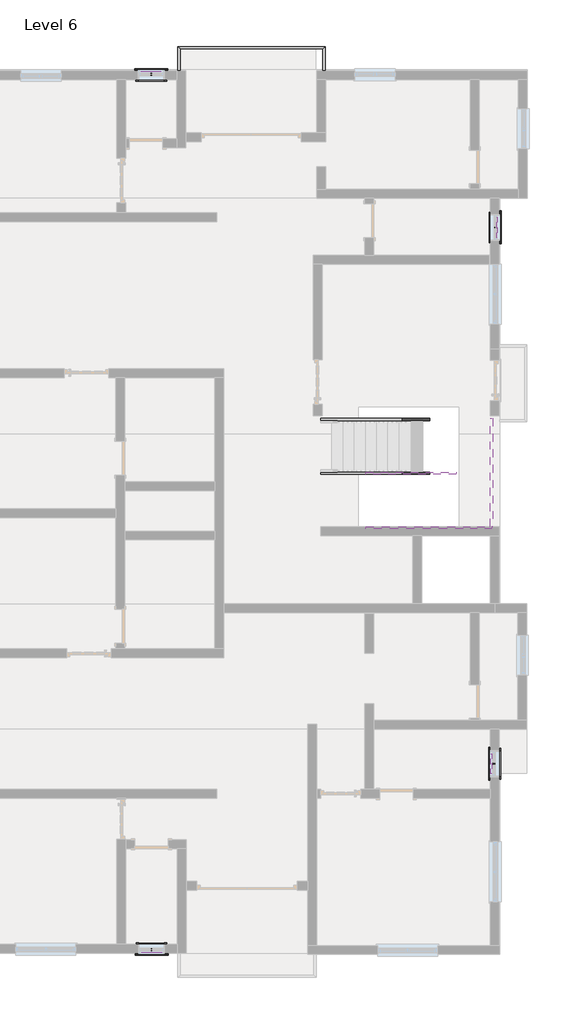
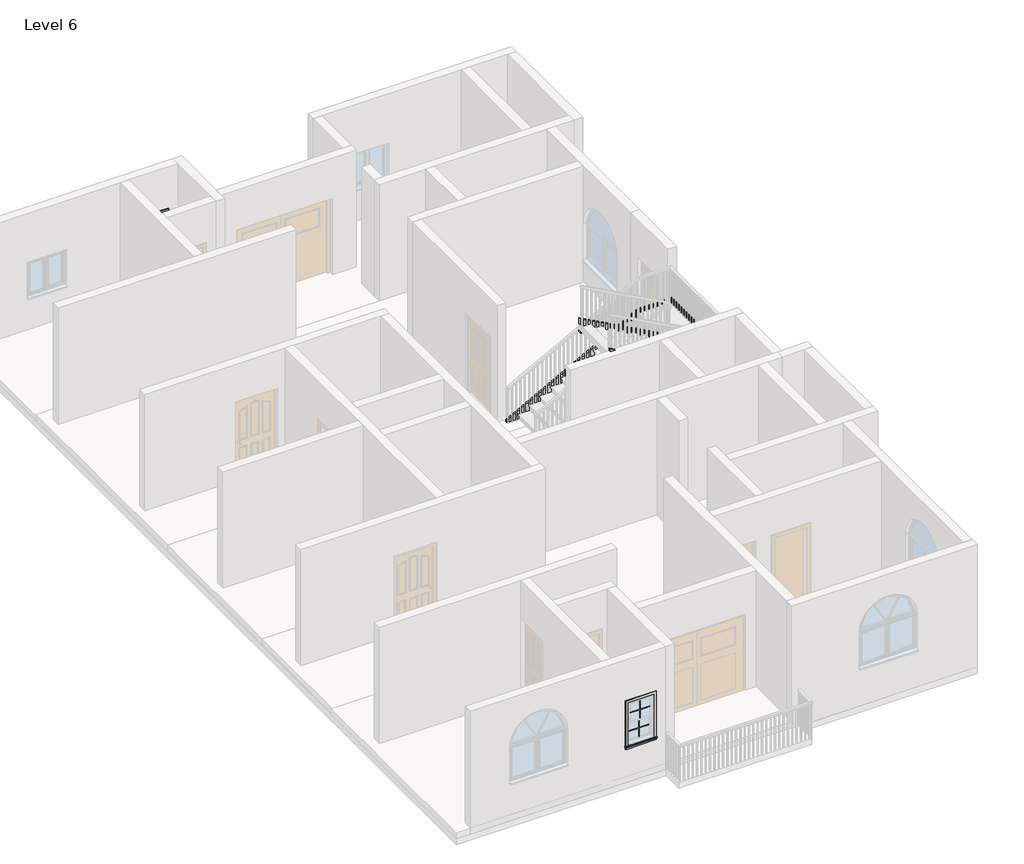
# One storey, part 7 of 7: 16 proxies, 5 members, 1 railing.
"""IFC4 building model written with IfcOpenShell, lengths in millimetres."""

from ifc_helpers import new_model, si_unit, frame, origin, place, context, project, spatial, polyline, outline, extrude, faceted_brep, transform, mapped, element, save
from components import muntin_pattern_2x2_muntin_pattern_2x2_eba6c5fb, trim_window_exterior_flat_with_sill_278e6a94, trim_window_interior_flat_picture_frame_e9fd5f45

model = new_model("IFC4")

# Units and contexts
model_context = context("Model", 3, world=origin())
ifc_project = project(units=[si_unit("LENGTHUNIT", "METRE", prefix="MILLI")], contexts=[model_context])

# Site, building, storey
site = spatial("IfcSite", under=ifc_project)
building = spatial("IfcBuilding", under=site)
storey = spatial("IfcBuildingStorey", under=building, Name="Level 6", Elevation=15240.0)

# Proxies
placement = place(None, origin())
muntin_pattern_2x2_muntin_pattern_2x2_shape = muntin_pattern_2x2_muntin_pattern_2x2_eba6c5fb(model_context)
element("IfcBuildingElementProxy", 1, Name="Muntin Pattern_2x2 : Muntin Pattern_2x2", ObjectType="Muntin Pattern_2x2 : Muntin Pattern_2x2", at=placement, inside=storey, context=model_context, shape_type="MappedRepresentation", body=[
    mapped(muntin_pattern_2x2_muntin_pattern_2x2_shape, transform((5828.2640963, 5846.2962251, 16710.025), x_axis=(0.0, -1.0, 0.0), y_axis=(1.0, 0.0, 0.0), z_axis=(0.0, 0.0, 1.0))),
])
element("IfcBuildingElementProxy", 2, Name="Muntin Pattern_2x2 : Muntin Pattern_2x2", ObjectType="Muntin Pattern_2x2 : Muntin Pattern_2x2", at=placement, inside=storey, context=model_context, shape_type="MappedRepresentation", body=[
    mapped(muntin_pattern_2x2_muntin_pattern_2x2_shape, transform((5783.8140963, 5846.2962251, 16230.6), x_axis=(0.0, -1.0, 0.0), y_axis=(1.0, 0.0, 0.0), z_axis=(0.0, 0.0, 1.0))),
])
element("IfcBuildingElementProxy", 3, Name="Muntin Pattern_2x2 : Muntin Pattern_2x2", ObjectType="Muntin Pattern_2x2 : Muntin Pattern_2x2", at=placement, inside=storey, context=model_context, shape_type="MappedRepresentation", body=[
    mapped(muntin_pattern_2x2_muntin_pattern_2x2_shape, transform((5694.9140963, -6313.9537749, 16710.025), x_axis=(0.0, 1.0, 0.0), y_axis=(-1.0, 0.0, 0.0), z_axis=(0.0, 0.0, 1.0))),
])
element("IfcBuildingElementProxy", 4, Name="Muntin Pattern_2x2 : Muntin Pattern_2x2", ObjectType="Muntin Pattern_2x2 : Muntin Pattern_2x2", at=placement, inside=storey, context=model_context, shape_type="MappedRepresentation", body=[
    mapped(muntin_pattern_2x2_muntin_pattern_2x2_shape, transform((5739.3640963, -6313.9537749, 16230.6), x_axis=(0.0, 1.0, 0.0), y_axis=(-1.0, 0.0, 0.0), z_axis=(0.0, 0.0, 1.0))),
])
element("IfcBuildingElementProxy", 5, Name="Muntin Pattern_2x2 : Muntin Pattern_2x2", ObjectType="Muntin Pattern_2x2 : Muntin Pattern_2x2", at=placement, inside=storey, context=model_context, shape_type="MappedRepresentation", body=[
    mapped(muntin_pattern_2x2_muntin_pattern_2x2_shape, transform((-2029.8609037, 9366.9277313, 16710.025), x_axis=(1.0, 0.0, 0.0), y_axis=(0.0, 1.0, 0.0), z_axis=(0.0, 0.0, 1.0))),
])
element("IfcBuildingElementProxy", 6, Name="Muntin Pattern_2x2 : Muntin Pattern_2x2", ObjectType="Muntin Pattern_2x2 : Muntin Pattern_2x2", at=placement, inside=storey, context=model_context, shape_type="MappedRepresentation", body=[
    mapped(muntin_pattern_2x2_muntin_pattern_2x2_shape, transform((-2029.8609037, 9322.4777313, 16230.6), x_axis=(1.0, 0.0, 0.0), y_axis=(0.0, 1.0, 0.0), z_axis=(0.0, 0.0, 1.0))),
])
element("IfcBuildingElementProxy", 7, Name="Muntin Pattern_2x2 : Muntin Pattern_2x2", ObjectType="Muntin Pattern_2x2 : Muntin Pattern_2x2", at=placement, inside=storey, context=model_context, shape_type="MappedRepresentation", body=[
    mapped(muntin_pattern_2x2_muntin_pattern_2x2_shape, transform((-2023.5109037, -10577.9787749, 16710.025), x_axis=(-1.0, 0.0, 0.0), y_axis=(0.0, -1.0, 0.0), z_axis=(0.0, 0.0, 1.0))),
])
element("IfcBuildingElementProxy", 8, Name="Muntin Pattern_2x2 : Muntin Pattern_2x2", ObjectType="Muntin Pattern_2x2 : Muntin Pattern_2x2", at=placement, inside=storey, context=model_context, shape_type="MappedRepresentation", body=[
    mapped(muntin_pattern_2x2_muntin_pattern_2x2_shape, transform((-2023.5109037, -10533.5287749, 16230.6), x_axis=(-1.0, 0.0, 0.0), y_axis=(0.0, -1.0, 0.0), z_axis=(0.0, 0.0, 1.0))),
])
trim_window_exterior_flat_with_sill_shape = trim_window_exterior_flat_with_sill_278e6a94(model_context)
element("IfcBuildingElementProxy", 9, Name="Trim-Window-Exterior-Flat : with Sill", ObjectType="Trim-Window-Exterior-Flat : with Sill", at=placement, inside=storey, context=model_context, shape_type="MappedRepresentation", body=[
    mapped(trim_window_exterior_flat_with_sill_shape, transform((5863.1890963, 5846.2962251, 17221.2), x_axis=(0.0, 1.0, 0.0), y_axis=(0.0, 0.0, 1.0), z_axis=(1.0, 0.0, 0.0))),
])
element("IfcBuildingElementProxy", 10, Name="Trim-Window-Exterior-Flat : with Sill", ObjectType="Trim-Window-Exterior-Flat : with Sill", at=placement, inside=storey, context=model_context, shape_type="MappedRepresentation", body=[
    mapped(trim_window_exterior_flat_with_sill_shape, transform((5659.9890963, -6313.9537749, 17221.2), x_axis=(0.0, -1.0, 0.0), y_axis=(0.0, 0.0, 1.0), z_axis=(-1.0, 0.0, 0.0))),
])
element("IfcBuildingElementProxy", 11, Name="Trim-Window-Exterior-Flat : with Sill", ObjectType="Trim-Window-Exterior-Flat : with Sill", at=placement, inside=storey, context=model_context, shape_type="MappedRepresentation", body=[
    mapped(trim_window_exterior_flat_with_sill_shape, transform((-2029.8609037, 9401.8527313, 17221.2), x_axis=(-1.0, 0.0, 0.0), y_axis=(0.0, 0.0, 1.0), z_axis=(0.0, 1.0, 0.0))),
])
element("IfcBuildingElementProxy", 12, Name="Trim-Window-Exterior-Flat : with Sill", ObjectType="Trim-Window-Exterior-Flat : with Sill", at=placement, inside=storey, context=model_context, shape_type="MappedRepresentation", body=[
    mapped(trim_window_exterior_flat_with_sill_shape, transform((-2023.5109037, -10612.9037749, 17221.2), x_axis=(1.0, 0.0, 0.0), y_axis=(0.0, 0.0, 1.0), z_axis=(0.0, -1.0, 0.0))),
])
trim_window_interior_flat_picture_frame_shape = trim_window_interior_flat_picture_frame_e9fd5f45(model_context)
element("IfcBuildingElementProxy", 13, Name="Trim-Window-Interior-Flat : Picture Frame", ObjectType="Trim-Window-Interior-Flat : Picture Frame", at=placement, inside=storey, context=model_context, shape_type="MappedRepresentation", body=[
    mapped(trim_window_interior_flat_picture_frame_shape, transform((5659.9890963, 5846.2962251, 17221.2), x_axis=(0.0, -1.0, 0.0), y_axis=(0.0, 0.0, 1.0), z_axis=(-1.0, 0.0, 0.0))),
])
element("IfcBuildingElementProxy", 14, Name="Trim-Window-Interior-Flat : Picture Frame", ObjectType="Trim-Window-Interior-Flat : Picture Frame", at=placement, inside=storey, context=model_context, shape_type="MappedRepresentation", body=[
    mapped(trim_window_interior_flat_picture_frame_shape, transform((5863.1890963, -6313.9537749, 17221.2), x_axis=(0.0, 1.0, 0.0), y_axis=(0.0, 0.0, 1.0), z_axis=(1.0, 0.0, 0.0))),
])
element("IfcBuildingElementProxy", 15, Name="Trim-Window-Interior-Flat : Picture Frame", ObjectType="Trim-Window-Interior-Flat : Picture Frame", at=placement, inside=storey, context=model_context, shape_type="MappedRepresentation", body=[
    mapped(trim_window_interior_flat_picture_frame_shape, transform((-2029.8609037, 9198.6527313, 17221.2), x_axis=(1.0, 0.0, 0.0), y_axis=(0.0, 0.0, 1.0), z_axis=(0.0, -1.0, 0.0))),
])
element("IfcBuildingElementProxy", 16, Name="Trim-Window-Interior-Flat : Picture Frame", ObjectType="Trim-Window-Interior-Flat : Picture Frame", at=placement, inside=storey, context=model_context, shape_type="MappedRepresentation", body=[
    mapped(trim_window_interior_flat_picture_frame_shape, transform((-2023.5109037, -10409.7037749, 17221.2), x_axis=(-1.0, 0.0, 0.0), y_axis=(0.0, 0.0, 1.0), z_axis=(0.0, 1.0, 0.0))),
])

# Members
element("IfcMember", 17, ObjectType="Stringer - 2\" Width", at=placement, inside=storey, context=model_context, shape_type="SweptSolid", body=[
    extrude(outline(polyline([(15447.4423129, 1811.8890963), (15240.0, 1811.8890963), (15240.0, 2068.9379367), (17117.2909091, 5536.6829612), (17117.2909091, 4896.4452154), (15447.4423129, 1811.8890963)])), frame((0.0, 1464.7962251, 0.0), z_axis=(0.0, 1.0, 0.0), x_axis=(0.0, 0.0, 1.0)), (0.0, 0.0, 1.0), 50.8),
])
element("IfcMember", 18, ObjectType="Stringer - 2\" Width", at=placement, inside=storey, context=model_context, shape_type="SweptSolid", body=[
    extrude(outline(polyline([(5659.9890963, 1515.5962251), (5710.7890963, 1515.5962251), (5710.7890963, -935.5037749), (5659.9890963, -935.5037749), (5659.9890963, 1515.5962251)])), frame((0.0, 0.0, 16812.4909091), z_axis=(0.0, 0.0, 1.0), x_axis=(1.0, 0.0, 0.0)), (0.0, 0.0, 1.0), 304.8),
])
element("IfcMember", 19, ObjectType="Stringer - 2\" Width", at=placement, inside=storey, context=model_context, shape_type="SweptSolid", body=[
    extrude(outline(polyline([(16812.4909091, 5687.6636359), (18354.0362324, 2827.8890963), (18007.7736638, 2827.8890963), (16812.4909091, 5045.2998579), (16812.4909091, 5687.6636359)])), frame((0.0, -986.3037749, 0.0), z_axis=(0.0, 1.0, 0.0), x_axis=(0.0, 0.0, 1.0)), (0.0, 0.0, 1.0), 50.8),
])
element("IfcMember", 20, ObjectType="Stringer - 2\" Width", at=placement, inside=storey, context=model_context, shape_type="SweptSolid", body=[
    extrude(outline(polyline([(15447.4423129, 1811.8890963), (15240.0, 1811.8890963), (15240.0, 2068.9379367), (16734.8485088, 4830.2326586), (17081.4462232, 4830.2326586), (15447.4423129, 1811.8890963)])), frame((0.0, 245.5962251, 0.0), z_axis=(0.0, 1.0, 0.0), x_axis=(0.0, 0.0, 1.0)), (0.0, 0.0, 1.0), 50.8),
])
element("IfcMember", 21, ObjectType="Stringer - 2\" Width", at=placement, inside=storey, context=model_context, shape_type="SweptSolid", body=[
    extrude(outline(polyline([(16901.0382157, 4881.0326586), (17247.3007843, 4881.0326586), (18354.0362324, 2827.8890963), (18007.7736638, 2827.8890963), (16901.0382157, 4881.0326586)])), frame((0.0, 245.5962251, 0.0), z_axis=(0.0, 1.0, 0.0), x_axis=(0.0, 0.0, 1.0)), (0.0, 0.0, 1.0), 50.8),
])

# Railing
element("IfcRailing", 22, ObjectType="Handrail - Rectangular", at=placement, inside=storey, context=model_context, shape_type="SolidModel", body=[
    faceted_brep([(-1426.6109037, 9402.2962251, 16154.4), (-1426.6109037, 9402.2962251, 16103.6), (-1375.8109037, 9402.2962251, 16103.6), (-1375.8109037, 9402.2962251, 16154.4), (-1426.6109037, 9948.3962251, 16154.4), (-1426.6109037, 9948.3962251, 16103.6), (-1375.8109037, 9897.5962251, 16103.6), (-1375.8109037, 9897.5962251, 16154.4), (1913.4890963, 9948.3962251, 16154.4), (1913.4890963, 9948.3962251, 16103.6), (1862.6890963, 9897.5962251, 16103.6), (1862.6890963, 9897.5962251, 16154.4), (1913.4890963, 9402.2962251, 16154.4), (1862.6890963, 9402.2962251, 16154.4), (1862.6890963, 9402.2962251, 16103.6), (1913.4890963, 9402.2962251, 16103.6)], [[[0, 1, 2, 3]], [[1, 0, 4, 5]], [[2, 1, 5, 6]], [[3, 2, 6, 7]], [[0, 3, 7, 4]], [[5, 4, 8, 9]], [[6, 5, 9, 10]], [[7, 6, 10, 11]], [[4, 7, 11, 8]], [[12, 13, 14, 15]], [[9, 8, 12, 15]], [[10, 9, 15, 14]], [[11, 10, 14, 13]], [[8, 11, 13, 12]]]),
    extrude(outline(polyline([(1878.5640963, 9424.5212251), (1897.6140963, 9424.5212251), (1897.6140963, 9405.4712251), (1878.5640963, 9405.4712251), (1878.5640963, 9424.5212251)])), frame((0.0, 0.0, 15240.0), z_axis=(0.0, 0.0, 1.0), x_axis=(1.0, 0.0, 0.0)), (0.0, 0.0, 1.0), 863.6),
    extrude(outline(polyline([(1878.5640963, 9526.1212251), (1897.6140963, 9526.1212251), (1897.6140963, 9507.0712251), (1878.5640963, 9507.0712251), (1878.5640963, 9526.1212251)])), frame((0.0, 0.0, 15240.0), z_axis=(0.0, 0.0, 1.0), x_axis=(1.0, 0.0, 0.0)), (0.0, 0.0, 1.0), 863.6),
    extrude(outline(polyline([(1878.5640963, 9627.7212251), (1897.6140963, 9627.7212251), (1897.6140963, 9608.6712251), (1878.5640963, 9608.6712251), (1878.5640963, 9627.7212251)])), frame((0.0, 0.0, 15240.0), z_axis=(0.0, 0.0, 1.0), x_axis=(1.0, 0.0, 0.0)), (0.0, 0.0, 1.0), 863.6),
    extrude(outline(polyline([(1878.5640963, 9729.3212251), (1897.6140963, 9729.3212251), (1897.6140963, 9710.2712251), (1878.5640963, 9710.2712251), (1878.5640963, 9729.3212251)])), frame((0.0, 0.0, 15240.0), z_axis=(0.0, 0.0, 1.0), x_axis=(1.0, 0.0, 0.0)), (0.0, 0.0, 1.0), 863.6),
    extrude(outline(polyline([(1878.5640963, 9830.9212251), (1897.6140963, 9830.9212251), (1897.6140963, 9811.8712251), (1878.5640963, 9811.8712251), (1878.5640963, 9830.9212251)])), frame((0.0, 0.0, 15240.0), z_axis=(0.0, 0.0, 1.0), x_axis=(1.0, 0.0, 0.0)), (0.0, 0.0, 1.0), 863.6),
    extrude(outline(polyline([(1840.4640963, 9913.4712251), (1840.4640963, 9932.5212251), (1859.5140963, 9932.5212251), (1859.5140963, 9913.4712251), (1840.4640963, 9913.4712251)])), frame((0.0, 0.0, 15240.0), z_axis=(0.0, 0.0, 1.0), x_axis=(1.0, 0.0, 0.0)), (0.0, 0.0, 1.0), 863.6),
    extrude(outline(polyline([(1738.8640963, 9913.4712251), (1738.8640963, 9932.5212251), (1757.9140963, 9932.5212251), (1757.9140963, 9913.4712251), (1738.8640963, 9913.4712251)])), frame((0.0, 0.0, 15240.0), z_axis=(0.0, 0.0, 1.0), x_axis=(1.0, 0.0, 0.0)), (0.0, 0.0, 1.0), 863.6),
    extrude(outline(polyline([(1637.2640963, 9913.4712251), (1637.2640963, 9932.5212251), (1656.3140963, 9932.5212251), (1656.3140963, 9913.4712251), (1637.2640963, 9913.4712251)])), frame((0.0, 0.0, 15240.0), z_axis=(0.0, 0.0, 1.0), x_axis=(1.0, 0.0, 0.0)), (0.0, 0.0, 1.0), 863.6),
    extrude(outline(polyline([(1535.6640963, 9913.4712251), (1535.6640963, 9932.5212251), (1554.7140963, 9932.5212251), (1554.7140963, 9913.4712251), (1535.6640963, 9913.4712251)])), frame((0.0, 0.0, 15240.0), z_axis=(0.0, 0.0, 1.0), x_axis=(1.0, 0.0, 0.0)), (0.0, 0.0, 1.0), 863.6),
    extrude(outline(polyline([(1434.0640963, 9913.4712251), (1434.0640963, 9932.5212251), (1453.1140963, 9932.5212251), (1453.1140963, 9913.4712251), (1434.0640963, 9913.4712251)])), frame((0.0, 0.0, 15240.0), z_axis=(0.0, 0.0, 1.0), x_axis=(1.0, 0.0, 0.0)), (0.0, 0.0, 1.0), 863.6),
    extrude(outline(polyline([(1332.4640963, 9913.4712251), (1332.4640963, 9932.5212251), (1351.5140963, 9932.5212251), (1351.5140963, 9913.4712251), (1332.4640963, 9913.4712251)])), frame((0.0, 0.0, 15240.0), z_axis=(0.0, 0.0, 1.0), x_axis=(1.0, 0.0, 0.0)), (0.0, 0.0, 1.0), 863.6),
    extrude(outline(polyline([(1230.8640963, 9913.4712251), (1230.8640963, 9932.5212251), (1249.9140963, 9932.5212251), (1249.9140963, 9913.4712251), (1230.8640963, 9913.4712251)])), frame((0.0, 0.0, 15240.0), z_axis=(0.0, 0.0, 1.0), x_axis=(1.0, 0.0, 0.0)), (0.0, 0.0, 1.0), 863.6),
    extrude(outline(polyline([(1129.2640963, 9913.4712251), (1129.2640963, 9932.5212251), (1148.3140963, 9932.5212251), (1148.3140963, 9913.4712251), (1129.2640963, 9913.4712251)])), frame((0.0, 0.0, 15240.0), z_axis=(0.0, 0.0, 1.0), x_axis=(1.0, 0.0, 0.0)), (0.0, 0.0, 1.0), 863.6),
    extrude(outline(polyline([(1027.6640963, 9913.4712251), (1027.6640963, 9932.5212251), (1046.7140963, 9932.5212251), (1046.7140963, 9913.4712251), (1027.6640963, 9913.4712251)])), frame((0.0, 0.0, 15240.0), z_axis=(0.0, 0.0, 1.0), x_axis=(1.0, 0.0, 0.0)), (0.0, 0.0, 1.0), 863.6),
    extrude(outline(polyline([(926.0640963, 9913.4712251), (926.0640963, 9932.5212251), (945.1140963, 9932.5212251), (945.1140963, 9913.4712251), (926.0640963, 9913.4712251)])), frame((0.0, 0.0, 15240.0), z_axis=(0.0, 0.0, 1.0), x_axis=(1.0, 0.0, 0.0)), (0.0, 0.0, 1.0), 863.6),
    extrude(outline(polyline([(824.4640963, 9913.4712251), (824.4640963, 9932.5212251), (843.5140963, 9932.5212251), (843.5140963, 9913.4712251), (824.4640963, 9913.4712251)])), frame((0.0, 0.0, 15240.0), z_axis=(0.0, 0.0, 1.0), x_axis=(1.0, 0.0, 0.0)), (0.0, 0.0, 1.0), 863.6),
    extrude(outline(polyline([(722.8640963, 9913.4712251), (722.8640963, 9932.5212251), (741.9140963, 9932.5212251), (741.9140963, 9913.4712251), (722.8640963, 9913.4712251)])), frame((0.0, 0.0, 15240.0), z_axis=(0.0, 0.0, 1.0), x_axis=(1.0, 0.0, 0.0)), (0.0, 0.0, 1.0), 863.6),
    extrude(outline(polyline([(621.2640963, 9913.4712251), (621.2640963, 9932.5212251), (640.3140963, 9932.5212251), (640.3140963, 9913.4712251), (621.2640963, 9913.4712251)])), frame((0.0, 0.0, 15240.0), z_axis=(0.0, 0.0, 1.0), x_axis=(1.0, 0.0, 0.0)), (0.0, 0.0, 1.0), 863.6),
    extrude(outline(polyline([(519.6640963, 9913.4712251), (519.6640963, 9932.5212251), (538.7140963, 9932.5212251), (538.7140963, 9913.4712251), (519.6640963, 9913.4712251)])), frame((0.0, 0.0, 15240.0), z_axis=(0.0, 0.0, 1.0), x_axis=(1.0, 0.0, 0.0)), (0.0, 0.0, 1.0), 863.6),
    extrude(outline(polyline([(418.0640963, 9913.4712251), (418.0640963, 9932.5212251), (437.1140963, 9932.5212251), (437.1140963, 9913.4712251), (418.0640963, 9913.4712251)])), frame((0.0, 0.0, 15240.0), z_axis=(0.0, 0.0, 1.0), x_axis=(1.0, 0.0, 0.0)), (0.0, 0.0, 1.0), 863.6),
    extrude(outline(polyline([(316.4640963, 9913.4712251), (316.4640963, 9932.5212251), (335.5140963, 9932.5212251), (335.5140963, 9913.4712251), (316.4640963, 9913.4712251)])), frame((0.0, 0.0, 15240.0), z_axis=(0.0, 0.0, 1.0), x_axis=(1.0, 0.0, 0.0)), (0.0, 0.0, 1.0), 863.6),
    extrude(outline(polyline([(214.8640963, 9913.4712251), (214.8640963, 9932.5212251), (233.9140963, 9932.5212251), (233.9140963, 9913.4712251), (214.8640963, 9913.4712251)])), frame((0.0, 0.0, 15240.0), z_axis=(0.0, 0.0, 1.0), x_axis=(1.0, 0.0, 0.0)), (0.0, 0.0, 1.0), 863.6),
    extrude(outline(polyline([(113.2640963, 9913.4712251), (113.2640963, 9932.5212251), (132.3140963, 9932.5212251), (132.3140963, 9913.4712251), (113.2640963, 9913.4712251)])), frame((0.0, 0.0, 15240.0), z_axis=(0.0, 0.0, 1.0), x_axis=(1.0, 0.0, 0.0)), (0.0, 0.0, 1.0), 863.6),
    extrude(outline(polyline([(11.6640963, 9913.4712251), (11.6640963, 9932.5212251), (30.7140963, 9932.5212251), (30.7140963, 9913.4712251), (11.6640963, 9913.4712251)])), frame((0.0, 0.0, 15240.0), z_axis=(0.0, 0.0, 1.0), x_axis=(1.0, 0.0, 0.0)), (0.0, 0.0, 1.0), 863.6),
    extrude(outline(polyline([(-89.9359037, 9913.4712251), (-89.9359037, 9932.5212251), (-70.8859037, 9932.5212251), (-70.8859037, 9913.4712251), (-89.9359037, 9913.4712251)])), frame((0.0, 0.0, 15240.0), z_axis=(0.0, 0.0, 1.0), x_axis=(1.0, 0.0, 0.0)), (0.0, 0.0, 1.0), 863.6),
    extrude(outline(polyline([(-191.5359037, 9913.4712251), (-191.5359037, 9932.5212251), (-172.4859037, 9932.5212251), (-172.4859037, 9913.4712251), (-191.5359037, 9913.4712251)])), frame((0.0, 0.0, 15240.0), z_axis=(0.0, 0.0, 1.0), x_axis=(1.0, 0.0, 0.0)), (0.0, 0.0, 1.0), 863.6),
    extrude(outline(polyline([(-293.1359037, 9913.4712251), (-293.1359037, 9932.5212251), (-274.0859037, 9932.5212251), (-274.0859037, 9913.4712251), (-293.1359037, 9913.4712251)])), frame((0.0, 0.0, 15240.0), z_axis=(0.0, 0.0, 1.0), x_axis=(1.0, 0.0, 0.0)), (0.0, 0.0, 1.0), 863.6),
    extrude(outline(polyline([(-394.7359037, 9913.4712251), (-394.7359037, 9932.5212251), (-375.6859037, 9932.5212251), (-375.6859037, 9913.4712251), (-394.7359037, 9913.4712251)])), frame((0.0, 0.0, 15240.0), z_axis=(0.0, 0.0, 1.0), x_axis=(1.0, 0.0, 0.0)), (0.0, 0.0, 1.0), 863.6),
    extrude(outline(polyline([(-496.3359037, 9913.4712251), (-496.3359037, 9932.5212251), (-477.2859037, 9932.5212251), (-477.2859037, 9913.4712251), (-496.3359037, 9913.4712251)])), frame((0.0, 0.0, 15240.0), z_axis=(0.0, 0.0, 1.0), x_axis=(1.0, 0.0, 0.0)), (0.0, 0.0, 1.0), 863.6),
    extrude(outline(polyline([(-597.9359037, 9913.4712251), (-597.9359037, 9932.5212251), (-578.8859037, 9932.5212251), (-578.8859037, 9913.4712251), (-597.9359037, 9913.4712251)])), frame((0.0, 0.0, 15240.0), z_axis=(0.0, 0.0, 1.0), x_axis=(1.0, 0.0, 0.0)), (0.0, 0.0, 1.0), 863.6),
    extrude(outline(polyline([(-699.5359037, 9913.4712251), (-699.5359037, 9932.5212251), (-680.4859037, 9932.5212251), (-680.4859037, 9913.4712251), (-699.5359037, 9913.4712251)])), frame((0.0, 0.0, 15240.0), z_axis=(0.0, 0.0, 1.0), x_axis=(1.0, 0.0, 0.0)), (0.0, 0.0, 1.0), 863.6),
    extrude(outline(polyline([(-801.1359037, 9913.4712251), (-801.1359037, 9932.5212251), (-782.0859037, 9932.5212251), (-782.0859037, 9913.4712251), (-801.1359037, 9913.4712251)])), frame((0.0, 0.0, 15240.0), z_axis=(0.0, 0.0, 1.0), x_axis=(1.0, 0.0, 0.0)), (0.0, 0.0, 1.0), 863.6),
    extrude(outline(polyline([(-902.7359037, 9913.4712251), (-902.7359037, 9932.5212251), (-883.6859037, 9932.5212251), (-883.6859037, 9913.4712251), (-902.7359037, 9913.4712251)])), frame((0.0, 0.0, 15240.0), z_axis=(0.0, 0.0, 1.0), x_axis=(1.0, 0.0, 0.0)), (0.0, 0.0, 1.0), 863.6),
    extrude(outline(polyline([(-1004.3359037, 9913.4712251), (-1004.3359037, 9932.5212251), (-985.2859037, 9932.5212251), (-985.2859037, 9913.4712251), (-1004.3359037, 9913.4712251)])), frame((0.0, 0.0, 15240.0), z_axis=(0.0, 0.0, 1.0), x_axis=(1.0, 0.0, 0.0)), (0.0, 0.0, 1.0), 863.6),
    extrude(outline(polyline([(-1105.9359037, 9913.4712251), (-1105.9359037, 9932.5212251), (-1086.8859037, 9932.5212251), (-1086.8859037, 9913.4712251), (-1105.9359037, 9913.4712251)])), frame((0.0, 0.0, 15240.0), z_axis=(0.0, 0.0, 1.0), x_axis=(1.0, 0.0, 0.0)), (0.0, 0.0, 1.0), 863.6),
    extrude(outline(polyline([(-1207.5359037, 9913.4712251), (-1207.5359037, 9932.5212251), (-1188.4859037, 9932.5212251), (-1188.4859037, 9913.4712251), (-1207.5359037, 9913.4712251)])), frame((0.0, 0.0, 15240.0), z_axis=(0.0, 0.0, 1.0), x_axis=(1.0, 0.0, 0.0)), (0.0, 0.0, 1.0), 863.6),
    extrude(outline(polyline([(-1309.1359037, 9913.4712251), (-1309.1359037, 9932.5212251), (-1290.0859037, 9932.5212251), (-1290.0859037, 9913.4712251), (-1309.1359037, 9913.4712251)])), frame((0.0, 0.0, 15240.0), z_axis=(0.0, 0.0, 1.0), x_axis=(1.0, 0.0, 0.0)), (0.0, 0.0, 1.0), 863.6),
    extrude(outline(polyline([(-1391.6859037, 9900.7712251), (-1410.7359037, 9900.7712251), (-1410.7359037, 9919.8212251), (-1391.6859037, 9919.8212251), (-1391.6859037, 9900.7712251)])), frame((0.0, 0.0, 15240.0), z_axis=(0.0, 0.0, 1.0), x_axis=(1.0, 0.0, 0.0)), (0.0, 0.0, 1.0), 863.6),
    extrude(outline(polyline([(-1391.6859037, 9799.1712251), (-1410.7359037, 9799.1712251), (-1410.7359037, 9818.2212251), (-1391.6859037, 9818.2212251), (-1391.6859037, 9799.1712251)])), frame((0.0, 0.0, 15240.0), z_axis=(0.0, 0.0, 1.0), x_axis=(1.0, 0.0, 0.0)), (0.0, 0.0, 1.0), 863.6),
    extrude(outline(polyline([(-1391.6859037, 9697.5712251), (-1410.7359037, 9697.5712251), (-1410.7359037, 9716.6212251), (-1391.6859037, 9716.6212251), (-1391.6859037, 9697.5712251)])), frame((0.0, 0.0, 15240.0), z_axis=(0.0, 0.0, 1.0), x_axis=(1.0, 0.0, 0.0)), (0.0, 0.0, 1.0), 863.6),
    extrude(outline(polyline([(-1391.6859037, 9595.9712251), (-1410.7359037, 9595.9712251), (-1410.7359037, 9615.0212251), (-1391.6859037, 9615.0212251), (-1391.6859037, 9595.9712251)])), frame((0.0, 0.0, 15240.0), z_axis=(0.0, 0.0, 1.0), x_axis=(1.0, 0.0, 0.0)), (0.0, 0.0, 1.0), 863.6),
    extrude(outline(polyline([(-1391.6859037, 9494.3712251), (-1410.7359037, 9494.3712251), (-1410.7359037, 9513.4212251), (-1391.6859037, 9513.4212251), (-1391.6859037, 9494.3712251)])), frame((0.0, 0.0, 15240.0), z_axis=(0.0, 0.0, 1.0), x_axis=(1.0, 0.0, 0.0)), (0.0, 0.0, 1.0), 863.6),
    extrude(outline(polyline([(1878.5640963, 9913.4712251), (1878.5640963, 9932.5212251), (1897.6140963, 9932.5212251), (1897.6140963, 9913.4712251), (1878.5640963, 9913.4712251)])), frame((0.0, 0.0, 15240.0), z_axis=(0.0, 0.0, 1.0), x_axis=(1.0, 0.0, 0.0)), (0.0, 0.0, 1.0), 863.6),
    extrude(outline(polyline([(-1391.6859037, 9913.4712251), (-1410.7359037, 9913.4712251), (-1410.7359037, 9932.5212251), (-1391.6859037, 9932.5212251), (-1391.6859037, 9913.4712251)])), frame((0.0, 0.0, 15240.0), z_axis=(0.0, 0.0, 1.0), x_axis=(1.0, 0.0, 0.0)), (0.0, 0.0, 1.0), 863.6),
    extrude(outline(polyline([(1878.5640963, 9421.3462251), (1897.6140963, 9421.3462251), (1897.6140963, 9402.2962251), (1878.5640963, 9402.2962251), (1878.5640963, 9421.3462251)])), frame((0.0, 0.0, 15240.0), z_axis=(0.0, 0.0, 1.0), x_axis=(1.0, 0.0, 0.0)), (0.0, 0.0, 1.0), 863.6),
    extrude(outline(polyline([(-1391.6859037, 9402.2962251), (-1410.7359037, 9402.2962251), (-1410.7359037, 9421.3462251), (-1391.6859037, 9421.3462251), (-1391.6859037, 9402.2962251)])), frame((0.0, 0.0, 15240.0), z_axis=(0.0, 0.0, 1.0), x_axis=(1.0, 0.0, 0.0)), (0.0, 0.0, 1.0), 863.6),
])

save(model, "model.ifc")

# Revit data of these elements
# Type "Muntin Pattern_2x2 : Muntin Pattern_2x2"
#   Width [instance default] = 4' - 0"
#   Thickness = 0' - 0 1/2"
#   Height [instance default] = 4' - 0"
#   Distance = 0' - 0 3/4"
#   Interior Material [instance default] = none
#   Exterior Material [instance default] = none
#   Default Elevation = 0
# Type "Trim-Window-Exterior-Flat : with Sill"
#   Trim Width = 0' - 2 1/4"
#   Trim Thickness_Picture Frame = 0' - 1 1/4"
#   Trim Thickness_with Sill = 0' - 0 3/4"
#   Sill Thickness = 0' - 1 1/4"
#   Opening Width [instance default] = 2' - 0"
#   Opening Height [instance default] = 3' - 0"
#   Default Elevation = 4' - 0"
#   Sill = yes
#   Picture Frame = no
#   Trim Material [instance default] = none
# Type "Trim-Window-Interior-Flat : Picture Frame"
#   Trim Thickness_Picture Frame = 0' - 1 1/4"
#   Trim Width = 0' - 2 1/4"
#   Trim Thickness_with Sill = 0' - 0 3/4"
#   Sill Thickness = 0' - 1 1/4"
#   Opening Width [instance default] = 2' - 0"
#   Opening Height [instance default] = 3' - 0"
#   Default Elevation = 4' - 0"
#   Sill = no
#   Picture Frame = yes
#   Trim Material [instance default] = none
# Type "Handrail - Rectangular"
#   Assembly Code = "C2010400"
#   built-in parameter 1008612 = 0.0416667 (stored number, unit not read)
#   built-in parameter 1008611 = 0.0416667 (stored number, unit not read)
#   built-in parameter 1008609 = 0.333333 (stored number, unit not read)
#   built-in parameter 1008604 = 0.166667 (stored number, unit not read)
#   built-in parameter 1008603 = 0.166667 (stored number, unit not read)
#   Railing Height = 3' - 0"
#   built-in parameter 1008630 = 2
#   built-in parameter 1008610 = 2
#   built-in parameter 1008618 = Baluster - Square : 3/4"
# Elements 1, 2, 3, 4, 5, 6, 7, 8 (IfcBuildingElementProxy, "Muntin Pattern_2x2 : Muntin Pattern_2x2")
#   Width = 1' - 6"
#   Height = 1' - 5 1/8"
#   Interior Material = Wood - Stained
#   Exterior Material = Clad - White
#   Phase Created = New Construction
#   Materials on its faces: "Clad - White", "Wood - Stained"
# Elements 9, 10, 11, 12 (IfcBuildingElementProxy, "Trim-Window-Exterior-Flat : with Sill")
#   Opening Width = 2' - 0"
#   Opening Height = 3' - 6"
#   Trim Material = Clad - White
#   Phase Created = New Construction
#   Materials on its faces: "Clad - White"
# Elements 13, 14, 15, 16 (IfcBuildingElementProxy, "Trim-Window-Interior-Flat : Picture Frame")
#   Opening Width = 2' - 0"
#   Opening Height = 3' - 6"
#   Trim Material = Wood - Stained
#   Phase Created = New Construction
#   Materials on its faces: "Wood - Stained"
# Elements 17, 18, 19, 20, 21 (IfcMember, "Stringer - 2\" Width")
#   Phase Created = New Construction
# Element 22 (IfcRailing, "Handrail - Rectangular")
#   Phase Created = New Construction
# Materials
#   "Clad - White": class "Wood", colour RGB 242 242 238, transparency 0, Cost = 0
#   "Wood - Stained": class "Wood", colour RGB 224 178 126, transparency 0, Cost = 0
